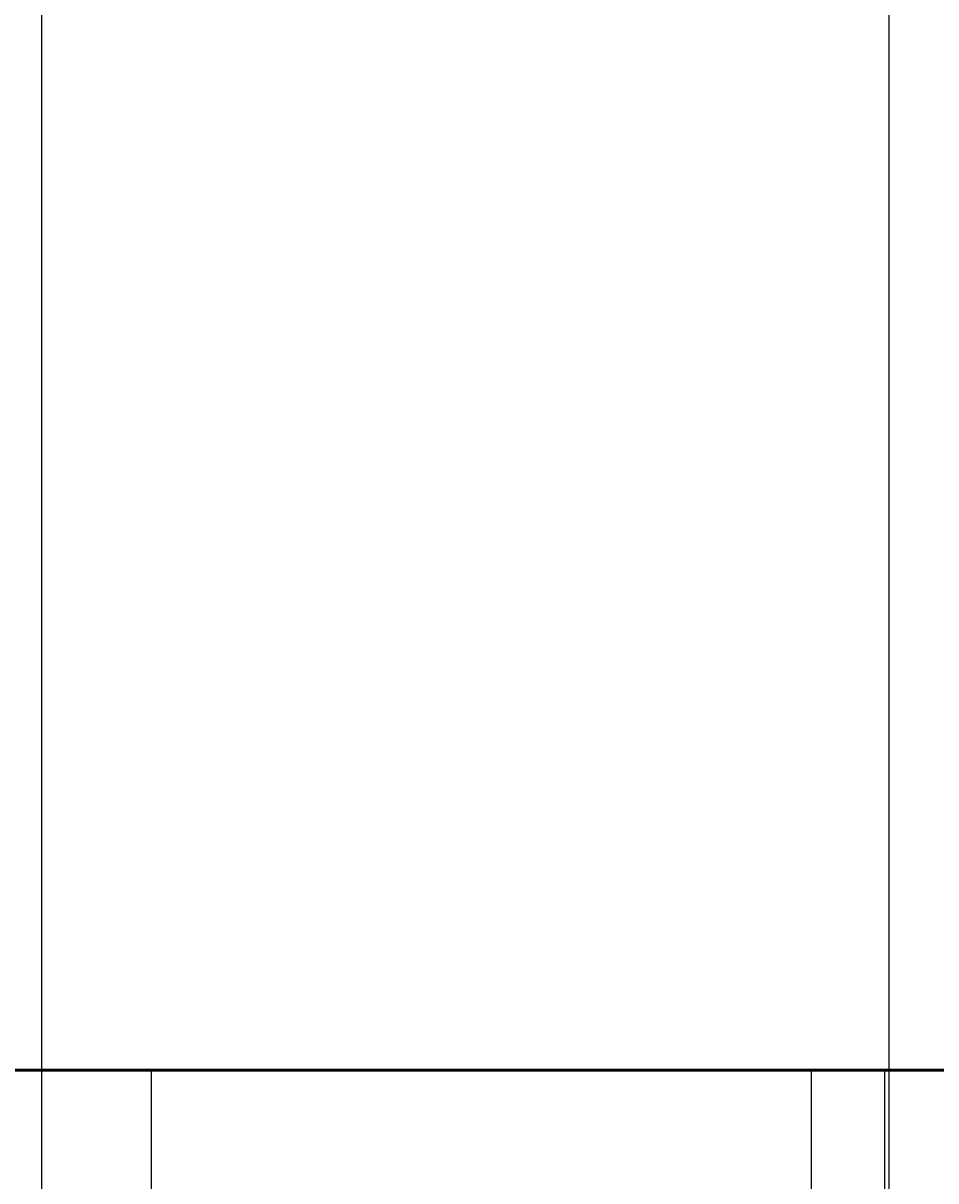
# Model space of a CAD drawing. Units: inches. Extents: x 37 to 824, y -700 to 234.
# Tile 30 of 77: x 227 to 251, y -269 to -237. Entities that reach past the tile are written whole.
import ezdxf

# ---------------------------------------------------------------- set-up
doc = ezdxf.new("R2010")
doc.units = ezdxf.units.IN
doc.header["$MEASUREMENT"] = 0
for name, color, linetype, lineweight in [('A-ANNO-DIMS', 2, 'Continuous', 18), ('A-GLAZ', 4, 'Continuous', 25), ('A-WALL', 2, 'Continuous', 50)]:
    doc.layers.add(name, color=color, linetype=linetype, lineweight=lineweight)
doc.styles.get("Standard").update_dxf_attribs({"font": 'arial.ttf'})
doc.dimstyles.get("Standard").update_dxf_attribs({"dimtxt": 0.18, "dimasz": 0.18, "dimexe": 0.18, "dimexo": 0.0625, "dimgap": 0.09, "dimtad": 0, "dimtih": 1, "dimtoh": 1, "dimdec": 1, "dimzin": 0, "dimdsep": 46, "dimlunit": 4, "dimtxsty": 'Standard', "dimcen": 0.09, "dimadec": 0, "dimazin": 0, "dimtfac": 1, "dimtdec": 1, "dimtofl": 0, "dimtmove": 0, "dimatfit": 3, "dimfxl": 1, "dimtolj": 1, "dimtzin": 0, "dimarcsym": 0})

# ---------------------------------------------------------------- blocks, each defined once
blk = doc.blocks.new('WIN-900')
for p, q in [((0, 9), (0, 0)), ((2, 9), (2, 0)), ((20, 9), (20, 0)), ((38, 9), (38, 0)), ((40, 9), (40, 0)), ((38, 5.5), (2, 5.5)), ((38, 3.5), (2, 3.5))]:
    blk.add_line(p, q)
blk = doc.blocks.new('*D77')
at = {"layer": 'A-ANNO-DIMS', "color": 0, "lineweight": -2, "ltscale": 0.5, "transparency": 16777216}
for p, q in [((227.077, 45.5), (227.077, -400.406)), ((290.077, 15.028), (290.077, -400.406)), ((227.257, -400.226), (258.248, -400.226)), ((289.897, -400.226), (258.906, -400.226))]:
    blk.add_line(p, q, dxfattribs=at)
at = {"layer": 'A-ANNO-DIMS', "color": 0, "ltscale": 0.5, "transparency": 16777216}
for points in [[(227.257, -400.196), (227.257, -400.256), (227.077, -400.226)], [(289.897, -400.196), (289.897, -400.256), (290.077, -400.226)]]:
    blk.add_solid(points, dxfattribs=at)
at = {"layer": 'Defpoints', "color": 0, "ltscale": 0.5, "transparency": 16777216}
for p in [(227.077, 45.563), (290.077, 15.09), (290.077, -400.226)]:
    blk.add_point(p, dxfattribs=at)
at = {"layer": 'A-ANNO-DIMS', "color": 0, "ltscale": 0.5, "transparency": 16777216, "insert": (258.577, -400.226), "char_height": 0.18, "attachment_point": 5}
blk.add_mtext('\\A1;5\'-3"', dxfattribs=at)
blk = doc.blocks.new('*D80')
at = {"layer": 'A-ANNO-DIMS', "color": 0, "lineweight": -2, "ltscale": 0.5, "transparency": 16777216}
for p, q in [((170.077, -167.972), (170.077, -400.406)), ((250.19, -167.972), (250.19, -400.406)), ((170.257, -400.226), (209.804, -400.226)), ((250.01, -400.226), (210.463, -400.226))]:
    blk.add_line(p, q, dxfattribs=at)
at = {"layer": 'A-ANNO-DIMS', "color": 0, "ltscale": 0.5, "transparency": 16777216}
for points in [[(170.257, -400.196), (170.257, -400.256), (170.077, -400.226)], [(250.01, -400.196), (250.01, -400.256), (250.19, -400.226)]]:
    blk.add_solid(points, dxfattribs=at)
at = {"layer": 'Defpoints', "color": 0, "ltscale": 0.5, "transparency": 16777216}
for p in [(170.077, -167.91), (250.19, -167.91), (250.19, -400.226)]:
    blk.add_point(p, dxfattribs=at)
at = {"layer": 'A-ANNO-DIMS', "color": 0, "ltscale": 0.5, "transparency": 16777216, "insert": (210.133, -400.226), "char_height": 0.18, "attachment_point": 5}
blk.add_mtext('\\A1;6\'-8"', dxfattribs=at)
blk = doc.blocks.new('*D81')
at = {"layer": 'A-ANNO-DIMS', "color": 0, "lineweight": -2, "ltscale": 0.5, "transparency": 16777216}
for p, q in [((290.077, -164.972), (290.077, -400.406)), ((250.19, -167.972), (250.19, -400.406)), ((250.37, -400.226), (269.804, -400.226)), ((289.897, -400.226), (270.463, -400.226))]:
    blk.add_line(p, q, dxfattribs=at)
at = {"layer": 'A-ANNO-DIMS', "color": 0, "ltscale": 0.5, "transparency": 16777216}
for points in [[(250.37, -400.196), (250.37, -400.256), (250.19, -400.226)], [(289.897, -400.196), (289.897, -400.256), (290.077, -400.226)]]:
    blk.add_solid(points, dxfattribs=at)
at = {"layer": 'Defpoints', "color": 0, "ltscale": 0.5, "transparency": 16777216}
for p in [(290.077, -164.91), (250.19, -167.91), (290.077, -400.226)]:
    blk.add_point(p, dxfattribs=at)
at = {"layer": 'A-ANNO-DIMS', "color": 0, "ltscale": 0.5, "transparency": 16777216, "insert": (270.133, -400.226), "char_height": 0.18, "attachment_point": 5}
blk.add_mtext('\\A1;3\'-4"', dxfattribs=at)
blk = doc.blocks.new('*D87')
at = {"layer": 'A-ANNO-DIMS', "color": 0, "lineweight": -2, "ltscale": 0.5, "transparency": 16777216}
for p, q in [((216.077, -356.847), (216.077, 234.17)), ((296.077, -356.847), (296.077, 234.17)), ((216.257, 233.99), (255.747, 233.99)), ((295.897, 233.99), (256.407, 233.99))]:
    blk.add_line(p, q, dxfattribs=at)
at = {"layer": 'A-ANNO-DIMS', "color": 0, "ltscale": 0.5, "transparency": 16777216}
for points in [[(216.257, 234.02), (216.257, 233.96), (216.077, 233.99)], [(295.897, 234.02), (295.897, 233.96), (296.077, 233.99)]]:
    blk.add_solid(points, dxfattribs=at)
at = {"layer": 'Defpoints', "color": 0, "ltscale": 0.5, "transparency": 16777216}
for p in [(296.077, 233.99), (216.077, -356.91), (296.077, -356.91)]:
    blk.add_point(p, dxfattribs=at)
at = {"layer": 'A-ANNO-DIMS', "color": 0, "ltscale": 0.5, "transparency": 16777216, "insert": (256.077, 233.99), "char_height": 0.18, "attachment_point": 5}
blk.add_mtext('\\A1;6\'-8"', dxfattribs=at)

msp = doc.modelspace()

# ---------------------------------------------------------------- linework, layer by layer
at = {"layer": 'A-WALL'}
msp.add_line((290.077, -265.91), (170.077, -265.91), dxfattribs=at)

# ---------------------------------------------------------------- block references
at = {"layer": 'A-GLAZ', "rotation": 180}
msp.add_blockref('WIN-900', (250.077, -265.909), dxfattribs=at)

# ---------------------------------------------------------------- dimensions: what is measured, and where the dimension line sits
at = {"layer": 'A-ANNO-DIMS', "ltscale": 0.5}
for base, p1, p2, picture, middle in [((296.077, 233.99), (216.077, -356.91), (296.077, -356.91), '*D87', (256.077, 233.99)), ((290.077, -400.226), (227.077, 45.563), (290.077, 15.09), '*D77', (258.577, -400.226)), ((290.077, -400.226), (250.19, -167.91), (290.077, -164.91), '*D81', (270.133, -400.226)), ((250.19, -400.226), (170.077, -167.91), (250.19, -167.91), '*D80', (210.133, -400.226))]:
    dim = msp.add_linear_dim(base=base, p1=p1, p2=p2, dimstyle='Standard', override={"dimdec": 1, "dimlfac": 1, "dimrnd": 0, "dimzin": 1, "dimdsep": 46, "dimlunit": 4, "dimfrac": 2}, dxfattribs=at)
    dim.commit()
    dim.dimension.update_dxf_attribs({"geometry": picture, "text_midpoint": middle})

doc.saveas('drawing.dxf')
